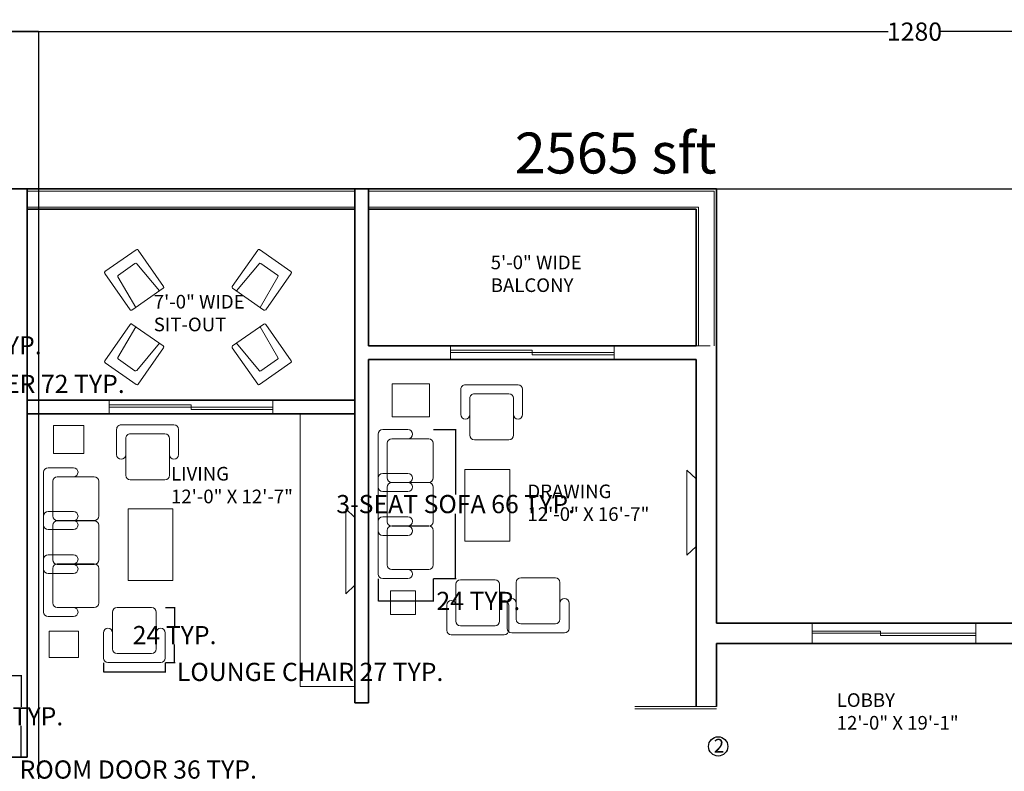
# Model space of a CAD drawing. Units: inches. Extents: x 3343 to 4790, y 1140 to 2641.
# Tile 6 of 10: x 3671 to 4104, y 2310 to 2641. Entities that reach past the tile are written whole.
import ezdxf

# ---------------------------------------------------------------- set-up
doc = ezdxf.new("R2010")
doc.units = ezdxf.units.IN
doc.header["$LTSCALE"] = 5
doc.header["$MEASUREMENT"] = 0
doc.linetypes.add('HIDDEN', pattern=[0.375, 0.25, -0.125])
for name, color, linetype, lineweight in [('A-ANNO-DIMS', 2, 'Continuous', 18), ('A-AREA-IDEN', 7, 'Continuous', 18), ('A-AREA-TAGS', 1, 'Continuous', 25), ('A-DOOR', 3, 'Continuous', 18), ('A-EQPM', 9, 'Continuous', 18), ('A-FLOR-CASE', 9, 'Continuous', 18), ('A-FLOR-HIDN', 8, 'HIDDEN', 13), ('A-FLOR-RAIL', 7, 'Continuous', 18), ('A-FURN', 8, 'Continuous', 13), ('A-GLAZ', 4, 'Continuous', 18), ('A-WALL', 7, 'Continuous', 35)]:
    doc.layers.add(name, color=color, linetype=linetype, lineweight=lineweight)
doc.styles.get("Standard").update_dxf_attribs({"font": 'arial.ttf'})
doc.dimstyles.get("Standard").update_dxf_attribs({"dimtxt": 8, "dimasz": 0.18, "dimexe": 0.18, "dimexo": 0.0625, "dimgap": 0.09, "dimtad": 0, "dimtih": 1, "dimtoh": 1, "dimdec": 1, "dimzin": 0, "dimdsep": 46, "dimlunit": 3, "dimtxsty": 'Standard', "dimcen": 0.09, "dimadec": 0, "dimazin": 0, "dimtfac": 1, "dimtdec": 1, "dimtofl": 0, "dimtmove": 0, "dimatfit": 3, "dimfxl": 1, "dimtolj": 1, "dimtzin": 0, "dimarcsym": 0})

# ---------------------------------------------------------------- blocks, each defined once
blk = doc.blocks.new('SOFA-3-SEAT')
for p, q in [((13.11, 65.51), (2, 65.51)), ((0, 63.51), (0, 40.3)), ((13.11, 61.51), (6, 61.51)), ((13.11, 61.51), (22.22, 61.51)), ((15.11, 63.51), (15.11, 63.51)), ((4, 59.51), (4, 44.3)), ((24.22, 44.3), (24.22, 59.51)), ((0, 44.2), (0, 20.98)), ((13.11, 46.2), (2, 46.2)), ((15.11, 44.2), (15.11, 44.2)), ((4, 40.2), (4, 24.98)), ((6, 42.3), (13.11, 42.3)), ((13.11, 42.2), (6, 42.2)), ((13.11, 42.3), (22.22, 42.3)), ((13.11, 42.2), (22.22, 42.2)), ((15.11, 40.3), (15.11, 40.3)), ((24.22, 24.98), (24.22, 40.2)), ((2, 38.3), (13.11, 38.3)), ((13.11, 27.21), (2, 27.21)), ((0, 25.21), (0, 2)), ((13.11, 23.21), (6, 23.21)), ((6, 22.98), (13.11, 22.98)), ((13.11, 23.21), (22.22, 23.21)), ((13.11, 22.98), (22.22, 22.98)), ((15.11, 25.21), (15.11, 25.21)), ((2, 18.98), (13.11, 18.98)), ((4, 21.21), (4, 6)), ((15.11, 20.98), (15.11, 20.98)), ((24.22, 6), (24.22, 21.21)), ((2, 0), (13.11, 0)), ((6, 4), (13.11, 4)), ((13.11, 4), (22.22, 4)), ((15.11, 2), (15.11, 2))]:
    blk.add_line(p, q)
for centre, start, end in [((2, 63.51), 90, 180), ((13.11, 63.51), 0, 90), ((6, 59.51), 90, 180), ((13.11, 63.51), 270, 0), ((22.22, 59.51), 0, 90), ((2, 44.2), 90, 180), ((6, 44.3), 180, 270), ((13.11, 44.2), 0, 90), ((13.11, 44.2), 270, 0), ((22.22, 44.3), 270, 0), ((2, 40.3), 180, 270), ((6, 40.2), 90, 180), ((13.11, 40.3), 0, 90), ((13.11, 40.3), 270, 0), ((22.22, 40.2), 0, 90), ((2, 25.21), 90, 180), ((13.11, 25.21), 0, 90), ((6, 24.98), 180, 270), ((6, 21.21), 90, 180), ((13.11, 25.21), 270, 0), ((13.11, 20.98), 0, 90), ((22.22, 24.98), 270, 0), ((22.22, 21.21), 0, 90), ((2, 20.98), 180, 270), ((13.11, 20.98), 270, 0), ((6, 6), 180, 270), ((22.22, 6), 270, 0), ((2, 2), 180, 270), ((13.11, 2), 0, 90), ((13.11, 2), 270, 0)]:
    blk.add_arc(centre, 2, start, end)
blk = doc.blocks.new('LOUNGE-CHAIR')
for p, q in [((4, 13.11), (4, 22.22)), ((6, 24.22), (21.21, 24.22)), ((23.21, 13.11), (23.21, 22.22)), ((0, 2), (0, 13.11)), ((2, 15.11), (2, 15.11)), ((4, 6), (4, 13.11)), ((23.21, 13.11), (23.21, 6)), ((25.21, 15.11), (25.21, 15.11)), ((27.21, 13.11), (27.21, 2)), ((21.21, 4), (6, 4)), ((25.21, 0), (2, 0))]:
    blk.add_line(p, q)
for centre, start, end in [((6, 22.22), 90, 180), ((21.21, 22.22), 0, 90), ((2, 13.11), 90, 180), ((2, 13.11), 0, 90), ((25.21, 13.11), 90, 180), ((25.21, 13.11), 0, 90), ((6, 6), 180, 270), ((21.21, 6), 270, 0), ((2, 2), 180, 270), ((25.21, 2), 270, 0)]:
    blk.add_arc(centre, 2, start, end)
blk = doc.blocks.new('CHAIR-SIDE')
for p, q in [((0, 0.6), (0, 20.1)), ((0.6, 20.7), (17.39, 20.7)), ((2.68, 20.7), (3.95, 5.17)), ((15.31, 20.7), (14.03, 5.17)), ((17.98, 20.1), (17.98, 0.6)), ((13.44, 4.62), (4.54, 4.62)), ((17.39, 0), (0.6, 0))]:
    blk.add_line(p, q)
for centre, start, end in [((0.6, 20.1), 90, 180), ((17.39, 20.1), 0, 90), ((4.54, 5.22), 184.6793, 270), ((13.44, 5.22), 270, 355.3207), ((0.6, 0.6), 180, 270), ((17.39, 0.6), 270, 0)]:
    blk.add_arc(centre, 0.595, start, end)
blk = doc.blocks.new('TV-WALL-MOUNT')
for p, q in [((0, 37.4), (4.02, 33.55)), ((0, 0), (4.02, 3.86))]:
    blk.add_line(p, q)
for points in [[(0, 37.4), (0, 0)], [(4.02, 0), (4.02, 37.4)]]:
    blk.add_lwpolyline(points)
blk = doc.blocks.new('WINDOW-72IN-SLIDING')
at = {"ltscale": 5}
for p, q in [((0, 6), (0, 0)), ((72, 6), (72, 0)), ((0, 4), (36, 4)), ((0, 3), (72, 3)), ((36, 4), (36, 2)), ((36, 2), (72, 2))]:
    blk.add_line(p, q, dxfattribs=at)
blk = doc.blocks.new('*D35')
at = {"layer": 'A-ANNO-DIMS', "color": 0, "lineweight": -2, "ltscale": 5, "transparency": 16777216}
for p, q in [((3707.6, 2357.71), (3707.6, 2353.52)), ((3734.82, 2357.71), (3734.82, 2353.52)), ((3707.78, 2353.7), (3734.64, 2353.7)), ((3734.82, 2353.7), (3735, 2353.7))]:
    blk.add_line(p, q, dxfattribs=at)
at = {"layer": 'A-ANNO-DIMS', "color": 0, "ltscale": 5, "transparency": 16777216}
for points in [[(3707.78, 2353.73), (3707.78, 2353.67), (3707.6, 2353.7)], [(3734.64, 2353.73), (3734.64, 2353.67), (3734.82, 2353.7)]]:
    blk.add_solid(points, dxfattribs=at)
at = {"layer": 'Defpoints', "color": 0, "ltscale": 5, "transparency": 16777216}
for p in [(3707.6, 2357.78), (3734.82, 2357.78), (3734.82, 2353.7)]:
    blk.add_point(p, dxfattribs=at)
at = {"layer": 'A-ANNO-DIMS', "color": 0, "ltscale": 5, "transparency": 16777216, "insert": (3798.47, 2353.7), "char_height": 8, "attachment_point": 5}
blk.add_mtext('\\A1;LOUNGE CHAIR 27 TYP.', dxfattribs=at)
blk = doc.blocks.new('*D36')
at = {"layer": 'A-ANNO-DIMS', "color": 0, "lineweight": -2, "ltscale": 5, "transparency": 16777216}
for p, q in [((3734.88, 2382), (3739.08, 2382)), ((3738.9, 2381.82), (3738.9, 2374)), ((3738.9, 2357.96), (3738.9, 2365.78)), ((3734.88, 2357.78), (3739.08, 2357.78))]:
    blk.add_line(p, q, dxfattribs=at)
at = {"layer": 'A-ANNO-DIMS', "color": 0, "ltscale": 5, "transparency": 16777216}
for points in [[(3738.87, 2381.82), (3738.93, 2381.82), (3738.9, 2382)], [(3738.87, 2357.96), (3738.93, 2357.96), (3738.9, 2357.78)]]:
    blk.add_solid(points, dxfattribs=at)
at = {"layer": 'Defpoints', "color": 0, "ltscale": 5, "transparency": 16777216}
for p in [(3734.82, 2382), (3738.9, 2382), (3734.82, 2357.78)]:
    blk.add_point(p, dxfattribs=at)
at = {"layer": 'A-ANNO-DIMS', "color": 0, "ltscale": 5, "transparency": 16777216, "insert": (3738.9, 2369.89), "char_height": 8, "attachment_point": 5}
blk.add_mtext('\\A1;24 TYP.', dxfattribs=at)
blk = doc.blocks.new('*D57')
at = {"layer": 'A-ANNO-DIMS', "color": 0, "lineweight": -2, "ltscale": 5, "transparency": 16777216}
for p, q in [((3852.67, 2460.26), (3862.61, 2460.26)), ((3862.43, 2460.08), (3862.43, 2431.74)), ((3862.43, 2394.93), (3862.43, 2423.28)), ((3852.67, 2394.75), (3862.61, 2394.75))]:
    blk.add_line(p, q, dxfattribs=at)
at = {"layer": 'A-ANNO-DIMS', "color": 0, "ltscale": 5, "transparency": 16777216}
for points in [[(3862.4, 2460.08), (3862.46, 2460.08), (3862.43, 2460.26)], [(3862.4, 2394.93), (3862.46, 2394.93), (3862.43, 2394.75)]]:
    blk.add_solid(points, dxfattribs=at)
at = {"layer": 'Defpoints', "color": 0, "ltscale": 5, "transparency": 16777216}
for p in [(3852.6, 2460.26), (3862.43, 2460.26), (3852.6, 2394.75)]:
    blk.add_point(p, dxfattribs=at)
at = {"layer": 'A-ANNO-DIMS', "color": 0, "ltscale": 5, "transparency": 16777216, "insert": (3862.43, 2427.51), "char_height": 8, "attachment_point": 5}
blk.add_mtext('\\A1;3-SEAT SOFA 66 TYP.', dxfattribs=at)
blk = doc.blocks.new('*D58')
at = {"layer": 'A-ANNO-DIMS', "color": 0, "lineweight": -2, "ltscale": 5, "transparency": 16777216}
for p, q in [((3828.38, 2394.69), (3828.38, 2384.74)), ((3852.6, 2394.69), (3852.6, 2384.74)), ((3828.56, 2384.92), (3852.42, 2384.92)), ((3852.6, 2384.92), (3852.78, 2384.92))]:
    blk.add_line(p, q, dxfattribs=at)
at = {"layer": 'A-ANNO-DIMS', "color": 0, "ltscale": 5, "transparency": 16777216}
for points in [[(3828.56, 2384.95), (3828.56, 2384.89), (3828.38, 2384.92)], [(3852.42, 2384.95), (3852.42, 2384.89), (3852.6, 2384.92)]]:
    blk.add_solid(points, dxfattribs=at)
at = {"layer": 'Defpoints', "color": 0, "ltscale": 5, "transparency": 16777216}
for p in [(3828.38, 2394.75), (3852.6, 2394.75), (3852.6, 2384.92)]:
    blk.add_point(p, dxfattribs=at)
at = {"layer": 'A-ANNO-DIMS', "color": 0, "ltscale": 5, "transparency": 16777216, "insert": (3872.41, 2384.92), "char_height": 8, "attachment_point": 5}
blk.add_mtext('\\A1;24 TYP.', dxfattribs=at)
blk = doc.blocks.new('*D61')
at = {"layer": 'A-ANNO-DIMS', "color": 0, "lineweight": -2, "ltscale": 5, "transparency": 16777216}
for p, q in [((3565.63, 2491.1), (3565.63, 2480.18)), ((3637.63, 2491.1), (3637.63, 2480.18)), ((3565.81, 2480.36), (3637.45, 2480.36)), ((3637.63, 2480.36), (3637.81, 2480.36))]:
    blk.add_line(p, q, dxfattribs=at)
at = {"layer": 'A-ANNO-DIMS', "color": 0, "ltscale": 5, "transparency": 16777216}
for points in [[(3565.81, 2480.39), (3565.81, 2480.33), (3565.63, 2480.36)], [(3637.45, 2480.39), (3637.45, 2480.33), (3637.63, 2480.36)]]:
    blk.add_solid(points, dxfattribs=at)
at = {"layer": 'Defpoints', "color": 0, "ltscale": 5, "transparency": 16777216}
for p in [(3565.63, 2491.16), (3637.63, 2491.16), (3637.63, 2480.36)]:
    blk.add_point(p, dxfattribs=at)
at = {"layer": 'A-ANNO-DIMS', "color": 0, "ltscale": 5, "transparency": 16777216, "insert": (3679.09, 2480.36), "char_height": 8, "attachment_point": 5}
blk.add_mtext('\\A1;SLIDER 72 TYP.', dxfattribs=at)
blk = doc.blocks.new('*D62')
at = {"layer": 'A-ANNO-DIMS', "color": 0, "lineweight": -2, "ltscale": 5, "transparency": 16777216}
for p, q in [((3648.43, 2497.16), (3648.43, 2497.34)), ((3648.43, 2497.34), (3648.61, 2497.34)), ((3637.69, 2497.16), (3648.61, 2497.16)), ((3648.43, 2491.34), (3648.43, 2496.98)), ((3637.69, 2491.16), (3648.61, 2491.16))]:
    blk.add_line(p, q, dxfattribs=at)
at = {"layer": 'A-ANNO-DIMS', "color": 0, "ltscale": 5, "transparency": 16777216}
for points in [[(3648.4, 2496.98), (3648.46, 2496.98), (3648.43, 2497.16)], [(3648.4, 2491.34), (3648.46, 2491.34), (3648.43, 2491.16)]]:
    blk.add_solid(points, dxfattribs=at)
at = {"layer": 'Defpoints', "color": 0, "ltscale": 5, "transparency": 16777216}
for p in [(3637.63, 2497.16), (3648.43, 2497.16), (3637.63, 2491.16)]:
    blk.add_point(p, dxfattribs=at)
at = {"layer": 'A-ANNO-DIMS', "color": 0, "ltscale": 5, "transparency": 16777216, "insert": (3665.08, 2497.34), "char_height": 8, "attachment_point": 5}
blk.add_mtext('\\A1;6 TYP.', dxfattribs=at)
blk = doc.blocks.new('*D65')
at = {"layer": 'A-ANNO-DIMS', "color": 0, "lineweight": -2, "ltscale": 5, "transparency": 16777216}
for p, q in [((3630.13, 2316.1), (3630.13, 2310.58)), ((3666.13, 2316.1), (3666.13, 2310.58)), ((3630.31, 2310.76), (3665.95, 2310.76)), ((3666.13, 2310.76), (3666.31, 2310.76))]:
    blk.add_line(p, q, dxfattribs=at)
at = {"layer": 'A-ANNO-DIMS', "color": 0, "ltscale": 5, "transparency": 16777216}
for points in [[(3630.31, 2310.79), (3630.31, 2310.73), (3630.13, 2310.76)], [(3665.95, 2310.79), (3665.95, 2310.73), (3666.13, 2310.76)]]:
    blk.add_solid(points, dxfattribs=at)
at = {"layer": 'Defpoints', "color": 0, "ltscale": 5, "transparency": 16777216}
for p in [(3630.13, 2316.16), (3666.13, 2316.16), (3666.13, 2310.76)]:
    blk.add_point(p, dxfattribs=at)
at = {"layer": 'A-ANNO-DIMS', "color": 0, "ltscale": 5, "transparency": 16777216, "insert": (3722.92, 2310.76), "char_height": 8, "attachment_point": 5}
blk.add_mtext('\\A1;ROOM DOOR 36 TYP.', dxfattribs=at)
blk = doc.blocks.new('*D66')
at = {"layer": 'A-ANNO-DIMS', "color": 0, "lineweight": -2, "ltscale": 5, "transparency": 16777216}
for p, q in [((3666.19, 2352.16), (3671.71, 2352.16)), ((3671.53, 2351.98), (3671.53, 2338.34)), ((3671.53, 2316.34), (3671.53, 2329.98)), ((3666.19, 2316.16), (3671.71, 2316.16))]:
    blk.add_line(p, q, dxfattribs=at)
at = {"layer": 'A-ANNO-DIMS', "color": 0, "ltscale": 5, "transparency": 16777216}
for points in [[(3671.5, 2351.98), (3671.56, 2351.98), (3671.53, 2352.16)], [(3671.5, 2316.34), (3671.56, 2316.34), (3671.53, 2316.16)]]:
    blk.add_solid(points, dxfattribs=at)
at = {"layer": 'Defpoints', "color": 0, "ltscale": 5, "transparency": 16777216}
for p in [(3666.13, 2352.16), (3671.53, 2352.16), (3666.13, 2316.16)]:
    blk.add_point(p, dxfattribs=at)
at = {"layer": 'A-ANNO-DIMS', "color": 0, "ltscale": 5, "transparency": 16777216, "insert": (3671.53, 2334.16), "char_height": 8, "attachment_point": 5}
blk.add_mtext('\\A1;36 TYP.', dxfattribs=at)
blk = doc.blocks.new('*D83')
at = {"layer": 'A-ANNO-DIMS', "color": 0, "lineweight": -2, "ltscale": 5, "transparency": 16777216}
for p, q in [((3424.13, 2432.05), (3424.13, 2635.49)), ((3424.31, 2635.31), (4052.48, 2635.31)), ((4703.95, 2635.31), (4075.77, 2635.31)), ((4704.13, 2197.22), (4704.13, 2635.49))]:
    blk.add_line(p, q, dxfattribs=at)
at = {"layer": 'A-ANNO-DIMS', "color": 0, "ltscale": 5, "transparency": 16777216}
for points in [[(3424.31, 2635.34), (3424.31, 2635.28), (3424.13, 2635.31)], [(4703.95, 2635.34), (4703.95, 2635.28), (4704.13, 2635.31)]]:
    blk.add_solid(points, dxfattribs=at)
at = {"layer": 'Defpoints', "color": 0, "ltscale": 5, "transparency": 16777216}
for p in [(4704.13, 2635.31), (3424.13, 2431.99), (4704.13, 2197.16)]:
    blk.add_point(p, dxfattribs=at)
at = {"layer": 'A-ANNO-DIMS', "color": 0, "ltscale": 5, "transparency": 16777216, "insert": (4064.13, 2635.31), "char_height": 8, "attachment_point": 5}
blk.add_mtext('\\A1;1280', dxfattribs=at)
blk = doc.blocks.new('*D84')
at = {"layer": 'A-ANNO-DIMS', "color": 0, "lineweight": -2, "ltscale": 5, "transparency": 16777216}
for p, q in [((3448.07, 2566.16), (3354.8, 2566.16)), ((3354.98, 2565.98), (3354.98, 1894.31)), ((3354.98, 1214.29), (3354.98, 1885.96)), ((4015.58, 1214.11), (3354.8, 1214.11))]:
    blk.add_line(p, q, dxfattribs=at)
at = {"layer": 'A-ANNO-DIMS', "color": 0, "ltscale": 5, "transparency": 16777216}
for points in [[(3354.95, 2565.98), (3355.01, 2565.98), (3354.98, 2566.16)], [(3354.95, 1214.29), (3355.01, 1214.29), (3354.98, 1214.11)]]:
    blk.add_solid(points, dxfattribs=at)
at = {"layer": 'Defpoints', "color": 0, "ltscale": 5, "transparency": 16777216}
for p in [(3448.13, 2566.16), (3354.98, 1214.11), (4015.65, 1214.11)]:
    blk.add_point(p, dxfattribs=at)
at = {"layer": 'A-ANNO-DIMS', "color": 0, "ltscale": 5, "transparency": 16777216, "insert": (3354.98, 1890.14), "char_height": 8, "attachment_point": 5}
blk.add_mtext('\\A1;1352', dxfattribs=at)
blk = doc.blocks.new('*D87')
at = {"layer": 'A-ANNO-DIMS', "color": 0, "lineweight": -2, "ltscale": 5, "transparency": 16777216}
for p, q in [((3977.19, 2566.16), (4773.46, 2566.16)), ((4773.28, 2565.98), (4773.28, 2294.34)), ((4773.28, 2014.34), (4773.28, 2285.99)), ((3977.19, 2014.16), (4773.46, 2014.16))]:
    blk.add_line(p, q, dxfattribs=at)
at = {"layer": 'A-ANNO-DIMS', "color": 0, "ltscale": 5, "transparency": 16777216}
for points in [[(4773.25, 2565.98), (4773.31, 2565.98), (4773.28, 2566.16)], [(4773.25, 2014.34), (4773.31, 2014.34), (4773.28, 2014.16)]]:
    blk.add_solid(points, dxfattribs=at)
at = {"layer": 'Defpoints', "color": 0, "ltscale": 5, "transparency": 16777216}
for p in [(3977.13, 2566.16), (3977.13, 2014.16), (4773.28, 2014.16)]:
    blk.add_point(p, dxfattribs=at)
at = {"layer": 'A-ANNO-DIMS', "color": 0, "ltscale": 5, "transparency": 16777216, "insert": (4773.28, 2290.16), "char_height": 8, "attachment_point": 5}
blk.add_mtext('\\A1;552', dxfattribs=at)
blk = doc.blocks.new('*D89')
at = {"layer": 'A-ANNO-DIMS', "color": 0, "lineweight": -2, "ltscale": 5, "transparency": 16777216}
for p, q in [((3977.19, 2566.16), (4773.46, 2566.16)), ((4773.28, 2565.98), (4773.28, 2507.84)), ((4773.28, 2441.34), (4773.28, 2499.49)), ((4121.19, 2441.16), (4773.46, 2441.16))]:
    blk.add_line(p, q, dxfattribs=at)
at = {"layer": 'A-ANNO-DIMS', "color": 0, "ltscale": 5, "transparency": 16777216}
for points in [[(4773.25, 2565.98), (4773.31, 2565.98), (4773.28, 2566.16)], [(4773.25, 2441.34), (4773.31, 2441.34), (4773.28, 2441.16)]]:
    blk.add_solid(points, dxfattribs=at)
at = {"layer": 'Defpoints', "color": 0, "ltscale": 5, "transparency": 16777216}
for p in [(3977.13, 2566.16), (4121.13, 2441.16), (4773.28, 2441.16)]:
    blk.add_point(p, dxfattribs=at)
at = {"layer": 'A-ANNO-DIMS', "color": 0, "ltscale": 5, "transparency": 16777216, "insert": (4773.28, 2503.66), "char_height": 8, "attachment_point": 5}
blk.add_mtext('\\A1;125', dxfattribs=at)
blk = doc.blocks.new('*D96')
at = {"layer": 'A-ANNO-DIMS', "color": 0, "lineweight": -2, "ltscale": 5, "transparency": 16777216}
for p, q in [((3619.25, 1835.73), (3619.25, 2635.49)), ((3619.43, 2635.31), (3643.42, 2635.31)), ((3679.07, 2635.31), (3655.08, 2635.31)), ((3679.25, 1835.73), (3679.25, 2635.49))]:
    blk.add_line(p, q, dxfattribs=at)
at = {"layer": 'A-ANNO-DIMS', "color": 0, "ltscale": 5, "transparency": 16777216}
for points in [[(3619.43, 2635.34), (3619.43, 2635.28), (3619.25, 2635.31)], [(3679.07, 2635.34), (3679.07, 2635.28), (3679.25, 2635.31)]]:
    blk.add_solid(points, dxfattribs=at)
at = {"layer": 'Defpoints', "color": 0, "ltscale": 5, "transparency": 16777216}
for p in [(3679.25, 2635.31), (3619.25, 1835.67), (3679.25, 1835.67)]:
    blk.add_point(p, dxfattribs=at)
at = {"layer": 'A-ANNO-DIMS', "color": 0, "ltscale": 5, "transparency": 16777216, "insert": (3649.25, 2635.31), "char_height": 8, "attachment_point": 5}
blk.add_mtext('\\A1;60', dxfattribs=at)

msp = doc.modelspace()

# ---------------------------------------------------------------- linework, layer by layer
at = {"layer": 'A-AREA-TAGS', "ltscale": 5}
msp.add_circle((3977.822, 2320.933), 4.235, dxfattribs=at)
at = {"layer": 'A-DOOR', "ltscale": 5}
for p, q in [((3977.13, 2338.46), (3941.13, 2338.46)), ((3977.13, 2337.46), (3941.13, 2337.46)), ((3977.13, 2338.46), (3968.13, 2338.46))]:
    msp.add_line(p, q, dxfattribs=at)
at = {"layer": 'A-FLOR-CASE'}
msp.add_line((3794.13, 2467.161), (3794.13, 2347.227), dxfattribs=at)
at = {"layer": 'A-FLOR-CASE', "ltscale": 5}
msp.add_line((3794.13, 2347.227), (3818.13, 2347.227), dxfattribs=at)
at = {"layer": 'A-FLOR-HIDN', "ltscale": 5}
msp.add_line((3968.13, 2497.161), (3977.13, 2497.161), dxfattribs=at)
at = {"layer": 'A-FLOR-RAIL', "ltscale": 5}
for p, q in [((3818.13, 2565.161), (3674.13, 2565.161)), ((3976.13, 2565.161), (3824.13, 2565.161)), ((3818.13, 2558.161), (3674.13, 2558.161)), ((3969.13, 2558.161), (3824.13, 2558.161))]:
    msp.add_line(p, q, dxfattribs=at)
at = {"layer": 'A-FLOR-RAIL'}
for p, q in [((3976.13, 2565.161), (3976.13, 2497.161)), ((3969.13, 2558.161), (3969.13, 2497.161))]:
    msp.add_line(p, q, dxfattribs=at)
at = {"layer": 'A-FURN', "ltscale": 5}
for points in [[(3834.607, 2480.389), (3850.893, 2480.389), (3850.893, 2465.932), (3834.607, 2465.932)], [(3685.666, 2462.104), (3699.036, 2462.104), (3699.036, 2449.79), (3685.666, 2449.79)], [(3866.429, 2442.783), (3886.283, 2442.783), (3886.283, 2411.151), (3866.429, 2411.151)], [(3718.505, 2425.364), (3738.055, 2425.364), (3738.055, 2393.963), (3718.505, 2393.963)], [(3833.78, 2389.294), (3844.729, 2389.294), (3844.729, 2378.945), (3833.78, 2378.945)], [(3683.733, 2371.665), (3696.65, 2371.665), (3696.65, 2359.984), (3683.733, 2359.984)]]:
    msp.add_lwpolyline(points, close=True, dxfattribs=at)
at = {"layer": 'A-GLAZ', "ltscale": 5}
for p, q in [((4019.13, 2375.161), (4019.13, 2366.161)), ((4091.13, 2375.161), (4091.13, 2366.161)), ((4049.13, 2371.661), (4019.13, 2371.661)), ((4091.13, 2370.661), (4019.13, 2370.661)), ((4049.13, 2371.661), (4049.13, 2369.661)), ((4091.13, 2369.661), (4049.13, 2369.661))]:
    msp.add_line(p, q, dxfattribs=at)
at = {"layer": 'A-WALL', "ltscale": 5}
for p, q in [((3977.13, 2566.161), (3448.13, 2566.161)), ((3818.13, 2557.161), (3674.13, 2557.161)), ((3968.13, 2557.161), (3824.13, 2557.161)), ((3968.13, 2497.161), (3824.13, 2497.161)), ((3968.13, 2491.161), (3824.13, 2491.161)), ((3818.13, 2473.161), (3674.13, 2473.161)), ((3818.13, 2467.161), (3674.13, 2467.161)), ((3824.13, 2340.161), (3818.13, 2340.161)), ((3674.13, 2316.161), (3666.13, 2316.161))]:
    msp.add_line(p, q, dxfattribs=at)
at = {"layer": 'A-WALL'}
for p, q in [((3674.13, 2566.161), (3674.13, 2316.161)), ((3818.13, 2566.161), (3818.13, 2340.161)), ((3824.13, 2566.161), (3824.13, 2497.161)), ((3977.13, 2566.161), (3977.13, 2375.161)), ((3968.13, 2557.161), (3968.13, 2497.161)), ((3824.13, 2491.161), (3824.13, 2340.161)), ((3968.13, 2491.161), (3968.13, 2338.46)), ((4121.13, 2375.161), (3977.13, 2375.161)), ((4121.13, 2366.161), (3977.13, 2366.161)), ((3977.13, 2366.161), (3977.13, 2338.46))]:
    msp.add_line(p, q, dxfattribs=at)

# ---------------------------------------------------------------- block references
at = {"layer": 'A-EQPM'}
for p in [(3964.111, 2405.019), (3814.111, 2388.054)]:
    msp.add_blockref('TV-WALL-MOUNT', p, dxfattribs=at)
at = {"layer": 'A-FURN'}
for name, p, rotation in [('CHAIR-SIDE', (3722.566, 2539.747), 214.9298811868687), ('CHAIR-SIDE', (3790.508, 2529.45), 145.0701188131325), ('CHAIR-SIDE', (3707.822, 2490.049), 325.0701188131308), ('CHAIR-SIDE', (3775.764, 2479.752), 34.92988118687217), ('LOUNGE-CHAIR', (3891.884, 2480.021), 180), ('LOUNGE-CHAIR', (3740.637, 2462.377), 180)]:
    msp.add_blockref(name, p, dxfattribs=dict(at, rotation=rotation))
for name, p in [('SOFA-3-SEAT', (3828.38, 2394.75)), ('SOFA-3-SEAT', (3681.336, 2378.012)), ('LOUNGE-CHAIR', (3858.537, 2370.011)), ('LOUNGE-CHAIR', (3885.078, 2370.845)), ('LOUNGE-CHAIR', (3707.603, 2357.777))]:
    msp.add_blockref(name, p, dxfattribs=at)
at = {"layer": 'A-GLAZ'}
for p in [(3860.13, 2491.161), (3710.13, 2467.161)]:
    msp.add_blockref('WINDOW-72IN-SLIDING', p, dxfattribs=at)

# ---------------------------------------------------------------- texts
at = {"layer": 'A-AREA-IDEN', "ltscale": 5, "char_height": 6, "attachment_point": 1}
for s, insert in [('5\'-0" WIDE \\PBALCONY', (3877.847, 2536.793)), ('7\'-0" WIDE\\PSIT-OUT', (3729.735, 2519.511)), ('LIVING\\P12\'-0" X 12\'-7"', (3737.316, 2443.864)), ('DRAWING\\P12\'-0" X 16\'-7"', (3893.983, 2436.105)), ('LOBBY\\P12\'-0" X 19\'-1"', (4029.924, 2344.308))]:
    msp.add_mtext_dynamic_manual_height_columns(s, width=189.69543, gutter_width=1, heights=[0], dxfattribs=dict(at, insert=insert))
at = {"layer": 'A-AREA-TAGS', "ltscale": 5, "attachment_point": 1}
for s, insert, char_height in [('2565 sft', (3888.396, 2590.912), 18), ('2', (3975.91, 2324.234), 6)]:
    msp.add_mtext_dynamic_manual_height_columns(s, width=189.69543, gutter_width=1, heights=[0], dxfattribs=dict(at, insert=insert, char_height=char_height))

# ---------------------------------------------------------------- dimensions: what is measured, and where the dimension line sits
at = {"layer": 'A-ANNO-DIMS', "ltscale": 5}
for base, p1, p2, picture, middle in [((4704.13, 2635.311), (3424.13, 2431.992), (4704.13, 2197.161), '*D83', (4064.13, 2635.311)), ((3679.248, 2635.311), (3619.248, 1835.669), (3679.248, 1835.669), '*D96', (3649.248, 2635.311))]:
    dim = msp.add_linear_dim(base=base, p1=p1, p2=p2, dimstyle='Standard', override={"dimdec": 0, "dimlfac": 1, "dimrnd": 0, "dimzin": 0, "dimdsep": 46, "dimlunit": 2}, dxfattribs=at)
    dim.commit()
    dim.dimension.update_dxf_attribs({"geometry": picture, "text_midpoint": middle})
for base, p1, p2, picture, middle in [((3354.98, 1214.112), (3448.13, 2566.161), (4015.647, 1214.112), '*D84', (3354.98, 1890.137)), ((4773.28, 2014.161), (3977.13, 2566.161), (3977.13, 2014.161), '*D87', (4773.28, 2290.161)), ((4773.28, 2441.161), (3977.13, 2566.161), (4121.13, 2441.161), '*D89', (4773.28, 2503.661))]:
    dim = msp.add_linear_dim(base=base, p1=p1, p2=p2, angle=90, dimstyle='Standard', override={"dimdec": 0, "dimlfac": 1, "dimrnd": 0, "dimzin": 0, "dimdsep": 46, "dimlunit": 2}, dxfattribs=at)
    dim.commit()
    dim.dimension.update_dxf_attribs({"geometry": picture, "text_midpoint": middle})
for base, p1, p2, text, picture, middle in [((3648.43, 2497.161), (3637.63, 2491.161), (3637.63, 2497.161), '<> TYP.', '*D62', (3665.084, 2497.341)), ((3862.43, 2460.265), (3852.603, 2394.751), (3852.603, 2460.265), '3-SEAT SOFA <> TYP.', '*D57', (3862.43, 2427.508)), ((3738.897, 2381.999), (3734.816, 2357.777), (3734.816, 2381.999), '<> TYP.', '*D36', (3738.897, 2369.888)), ((3671.53, 2352.161), (3666.13, 2316.161), (3666.13, 2352.161), '<> TYP.', '*D66', (3671.53, 2334.161))]:
    dim = msp.add_linear_dim(base=base, p1=p1, p2=p2, angle=90, text=text, dimstyle='Standard', override={"dimdec": 0, "dimlfac": 1, "dimrnd": 0, "dimzin": 0, "dimdsep": 46, "dimlunit": 2}, dxfattribs=at)
    dim.commit()
    dim.dimension.update_dxf_attribs({"geometry": picture, "text_midpoint": middle})
for base, p1, p2, text, picture, middle in [((3637.63, 2480.361), (3565.63, 2491.161), (3637.63, 2491.161), 'SLIDER <> TYP.', '*D61', (3679.089, 2480.361)), ((3852.603, 2384.923), (3828.38, 2394.751), (3852.603, 2394.751), '<> TYP.', '*D58', (3872.412, 2384.923)), ((3734.816, 2353.695), (3707.603, 2357.777), (3734.816, 2357.777), 'LOUNGE CHAIR <> TYP.', '*D35', (3798.469, 2353.695)), ((3666.13, 2310.761), (3630.13, 2316.161), (3666.13, 2316.161), 'ROOM DOOR <> TYP.', '*D65', (3722.915, 2310.761))]:
    dim = msp.add_linear_dim(base=base, p1=p1, p2=p2, text=text, dimstyle='Standard', override={"dimdec": 0, "dimlfac": 1, "dimrnd": 0, "dimzin": 0, "dimdsep": 46, "dimlunit": 2}, dxfattribs=at)
    dim.commit()
    dim.dimension.update_dxf_attribs({"geometry": picture, "text_midpoint": middle})

doc.saveas('drawing.dxf')
